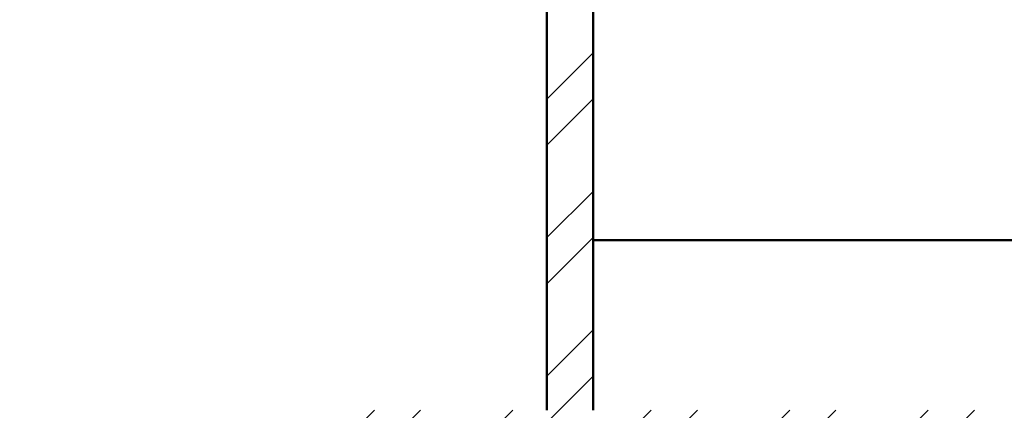
# Model space of a CAD drawing. Units: inches. Extents: x 963 to 2075, y 289 to 2657.
# Tile 36 of 98: x 1594 to 1689, y 1547 to 1585. Entities that reach past the tile are written whole.
import ezdxf

# ---------------------------------------------------------------- set-up
doc = ezdxf.new("R2010")
doc.units = ezdxf.units.IN
doc.layers.add('A-WALL', color=7, linetype='Continuous', lineweight=50)
doc.layers.add('A-WALL-PATT', color=8, linetype='Continuous', lineweight=13)

msp = doc.modelspace()

# ---------------------------------------------------------------- hatches: boundary and pattern name
at = {"layer": 'A-WALL-PATT'}
h = msp.add_hatch(dxfattribs=at)
h.set_pattern_fill('ANSI32', color=256)
h.paths.add_polyline_path([(1910.422, 1929.422), (1910.422, 1963.511), (1905.922, 1963.511), (1905.922, 1929.422), (1845.922, 1929.422), (1845.922, 1993.365), (1843.672, 1993.365), (1841.422, 1993.365), (1841.422, 1951.163), (1841.422, 1924.922), (1853.422, 1924.922), (1853.422, 1913.074), (1857.922, 1913.074), (1857.922, 1924.922), (1910.422, 1924.922)])
h.paths.add_polyline_path([(1857.922, 1853.074), (1853.422, 1853.074), (1853.422, 1826.318), (1841.422, 1826.318), (1674.482, 1826.318), (1674.482, 1821.818), (1853.422, 1821.818), (1857.922, 1821.818)])
h.paths.add_polyline_path([(1857.922, 1821.818), (1853.422, 1821.818), (1853.422, 1807.793), (1857.922, 1807.793)])
h.paths.add_polyline_path([(1857.922, 1747.793), (1853.422, 1747.793), (1853.422, 1713.818), (1809.343, 1713.818), (1809.343, 1709.318), (1905.922, 1709.318), (1905.922, 1688.318), (1910.422, 1688.318), (1910.422, 1713.818), (1857.922, 1713.818)])
h.paths.add_polyline_path([(1830.922, 1542.818), (1837.429, 1542.818), (1837.429, 1545.068), (1837.429, 1547.318), (1823.419, 1547.318), (1823.419, 1545.068), (1823.419, 1542.818), (1826.422, 1542.818), (1826.422, 1482.818), (1742.422, 1482.818), (1742.422, 1505.389), (1737.922, 1505.389), (1737.922, 1478.318), (1830.922, 1478.318)])
h.paths.add_polyline_path([(1938.922, 1619.318), (1934.422, 1619.318), (1910.422, 1619.318), (1910.422, 1628.318), (1908.172, 1628.318), (1905.922, 1628.318), (1905.922, 1614.818), (1934.422, 1614.818), (1934.422, 1547.318), (1905.922, 1547.318), (1899.589, 1547.318), (1899.589, 1542.818), (1910.422, 1542.818), (1938.922, 1542.818)])
h.paths.add_polyline_path([(1803.676, 1547.318), (1773.922, 1547.318), (1773.922, 1709.318), (1777.757, 1709.318), (1777.757, 1713.818), (1701.922, 1713.818), (1701.922, 1697.802), (1706.422, 1697.802), (1706.422, 1709.318), (1769.422, 1709.318), (1769.422, 1662.818), (1706.422, 1662.818), (1706.422, 1674.385), (1701.922, 1674.385), (1701.922, 1662.818), (1675.672, 1662.818), (1675.672, 1658.318), (1769.422, 1658.318), (1769.422, 1547.318), (1729.17, 1547.318), (1729.17, 1542.818), (1737.922, 1542.818), (1737.922, 1529.389), (1742.422, 1529.389), (1742.422, 1542.818), (1803.676, 1542.818)])
h.paths.add_polyline_path([(1595.422, 1542.818), (1599.245, 1542.818), (1599.245, 1547.318), (1584.36, 1547.318), (1584.36, 1542.818), (1590.922, 1542.818), (1590.922, 1436.318), (1595.422, 1436.318), (1595.422, 1440.818)])
h.paths.add_polyline_path([(1693.17, 1547.318), (1649.422, 1547.318), (1649.422, 1658.318), (1652.098, 1658.318), (1652.098, 1660.568), (1652.098, 1662.818), (1649.422, 1662.818), (1649.422, 1680.937), (1647.172, 1680.937), (1644.922, 1680.937), (1644.922, 1547.318), (1622.422, 1547.318), (1622.422, 1545.068), (1622.422, 1542.818), (1649.422, 1542.818), (1679.422, 1542.818), (1679.422, 1529.845), (1681.672, 1529.845), (1683.922, 1529.845), (1683.922, 1542.818), (1693.17, 1542.818), (1693.17, 1545.068)])
h.paths.add_polyline_path([(1683.922, 1505.845), (1679.422, 1505.845), (1679.422, 1483.805), (1595.422, 1483.805), (1595.422, 1479.305), (1683.922, 1479.305)])
h.paths.add_polyline_path([(1402.993, 1547.318), (1376.422, 1547.318), (1376.422, 1675.888), (1374.172, 1675.888), (1371.922, 1675.888), (1371.922, 1662.818), (1368.876, 1662.818), (1368.876, 1658.318), (1371.922, 1658.318), (1371.922, 1547.318), (1335.464, 1547.318), (1335.464, 1542.818), (1337.422, 1542.818), (1337.422, 1526.732), (1341.922, 1526.732), (1341.922, 1542.818), (1371.922, 1542.818), (1402.993, 1542.818)])

# ---------------------------------------------------------------- linework, layer by layer
at = {"layer": 'A-WALL'}
for p, q in [((1644.922, 1547.318), (1644.922, 1681.984)), ((1649.422, 1547.318), (1649.422, 1658.318)), ((1751.392, 1563.868), (1649.422, 1563.868))]:
    msp.add_line(p, q, dxfattribs=at)

doc.saveas('drawing.dxf')
